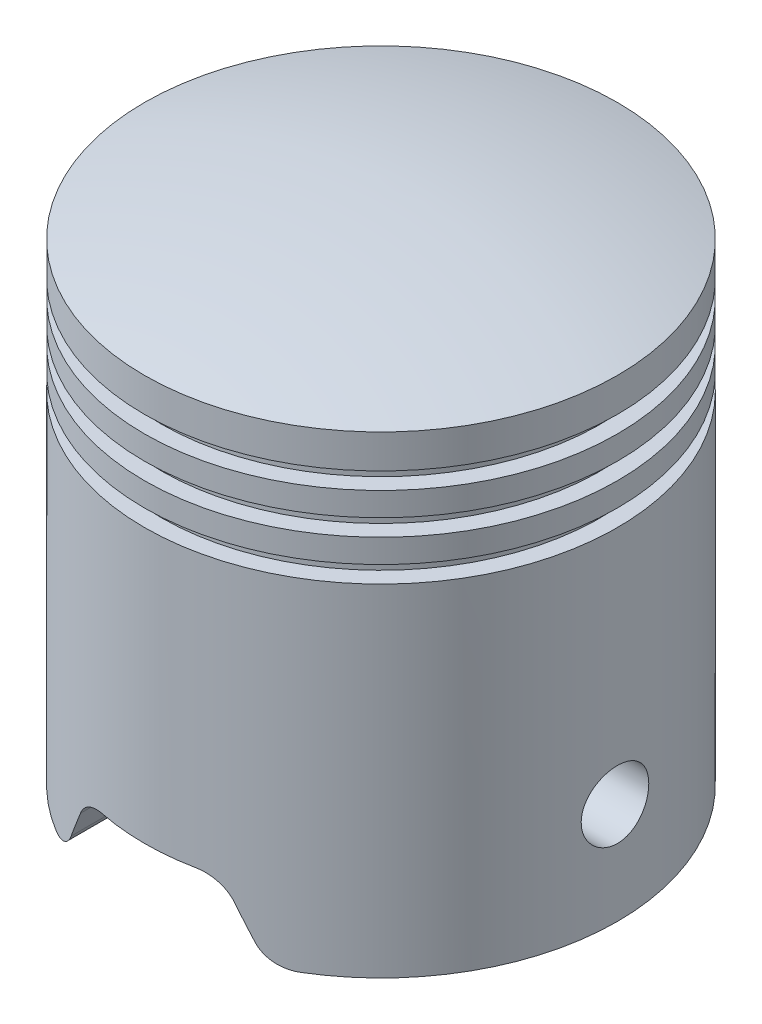
from build123d import *

# Parameters (mm, degrees)
PISTON_BODY_SKETCH_R       = 35
PISTON_BODY_70_DEPTH       = 35
RING_GROOVES_SKETCH_W      = 2.5
RING_GROOVES_SKETCH_H      = 2.5
INNER_BORE_SKETCH_R        = 29
INNER_BORE_58_DEPTH        = 65
SKIRT_CUTOUTS_DEPTH        = 61.621778265
SKIRT_CUTOUTS_DEPTH_BACK   = 61.621778265
SKIRT_CUTOUT_FILLET_R5_R   = 5
PIN_HOLE_10_DEPTH          = 61.621778438
PIN_HOLE_10_DEPTH_BACK     = 61.621778438
PIN_HOLE_SKETCH_R          = 5
PIN_BOSS_SKETCH_R          = 7.5
PIN_BOSS_15_DEPTH          = 32.5
PIN_BORE_DEPTH             = 84.703345378
PIN_BORE_DEPTH_BACK        = 84.703345378
PIN_BORE_SKETCH_R          = 5
CROWN_DOME_5MM_FACE_RADIUS = 35
CROWN_DOME_5MM_HEIGHT      = 5


with BuildPart() as part:
    # Piston Body Sketch → Piston Body _70 (new, symmetric)
    with BuildSketch(Plane(origin=(0, 0, 0), x_dir=(1, 0, 0), z_dir=(0, 1, 0))):
        with Locations(Location((0, 0, 0), (0, 0, 270))):
            Circle(PISTON_BODY_SKETCH_R)
    extrude(amount=PISTON_BODY_70_DEPTH, both=True)

    # Ring Grooves Sketch → Ring Grooves (revolve, cut)
    with BuildSketch(Plane(origin=(0, 0, 0), x_dir=(0, 0, -1), z_dir=(1, 0, 0))):
        with Locations((-33.75, 28.75)):
            Rectangle(RING_GROOVES_SKETCH_W, RING_GROOVES_SKETCH_H)
        with Locations((-33.75, 22.75)):
            Rectangle(RING_GROOVES_SKETCH_W, RING_GROOVES_SKETCH_H)
        with Locations((-33.75, 16.75)):
            Rectangle(RING_GROOVES_SKETCH_W, RING_GROOVES_SKETCH_H)
    revolve(axis=Axis((0, 35, 0), (0, -1, 0)), mode=Mode.SUBTRACT)

    # Inner Bore Sketch → Inner Bore _58 (cut)
    with BuildSketch(Plane.XZ.offset(35)):
        with Locations(Location((0, 0, 0), (0, 0, 270))):
            Circle(INNER_BORE_SKETCH_R)
    extrude(amount=-INNER_BORE_58_DEPTH, mode=Mode.SUBTRACT)

    # Skirt Cutout Sketch → Skirt Cutouts (cut, two sides: drawn at the far end of the back side and taken through both)
    with BuildSketch(Plane.XY.offset(-SKIRT_CUTOUTS_DEPTH_BACK)):
        with BuildLine():
            Line((15, -35), (-15, -35))
            Line((-15, -35), (-11.381966011, -27.763932023))
            ThreePointArc((-11.381966011, -27.763932023), (-9.538485617, -25.746745958), (-6.909830056, -25))
            Line((-6.909830056, -25), (6.909830056, -25))
            ThreePointArc((6.909830056, -25), (9.538485617, -25.746745958), (11.381966011, -27.763932023))
            Line((11.381966011, -27.763932023), (15, -35))
        make_face()
    extrude(amount=SKIRT_CUTOUTS_DEPTH + SKIRT_CUTOUTS_DEPTH_BACK, mode=Mode.SUBTRACT)

    # Skirt Cutout Fillet R5
    skirt_cutout_fillet_r5_edges = [part.edges().sort_by_distance(p)[0] for p in [
        (15, -35, -28.221061947),
        (15, -35, 28.221061947),
        (-15, -35, -28.221061947),
        (-15, -35, 28.221061947),
    ]]
    fillet(skirt_cutout_fillet_r5_edges, radius=SKIRT_CUTOUT_FILLET_R5_R)

    # Pin Hole Sketch → Pin Hole _10 (cut, two sides: drawn at the far end of the back side and taken through both)
    with BuildSketch(Plane(origin=(0, 0, 0), x_dir=(0, 0, -1), z_dir=(1, 0, 0)).offset(-PIN_HOLE_10_DEPTH_BACK)):
        with Locations((0, -20)):
            Circle(PIN_HOLE_SKETCH_R)
    extrude(amount=PIN_HOLE_10_DEPTH + PIN_HOLE_10_DEPTH_BACK, mode=Mode.SUBTRACT)

    # Pin Boss Sketch → Pin Boss _15 (add, symmetric)
    with BuildSketch(Plane(origin=(0, 0, 0), x_dir=(0, 0, -1), z_dir=(1, 0, 0))):
        with Locations(Location((0, -20, 0), (0, 0, 180))):
            Circle(PIN_BOSS_SKETCH_R)
    extrude(amount=PIN_BOSS_15_DEPTH, both=True)

    # Pin Bore Sketch → Pin Bore (cut, two sides: drawn at the far end of the back side and taken through both)
    with BuildSketch(Plane(origin=(32.5, 0, 0), x_dir=(0, 0, -1), z_dir=(1, 0, 0)).offset(-PIN_BORE_DEPTH_BACK)):
        with Locations((0, -20)):
            Circle(PIN_BORE_SKETCH_R)
    extrude(amount=PIN_BORE_DEPTH + PIN_BORE_DEPTH_BACK, mode=Mode.SUBTRACT)

    # Crown Dome 5mm: a dome of height H over a round flat face of radius A is a cap of a sphere of radius (A * A + H * H) / (2 * H)
    crown_dome_5mm_r = (CROWN_DOME_5MM_FACE_RADIUS * CROWN_DOME_5MM_FACE_RADIUS + CROWN_DOME_5MM_HEIGHT * CROWN_DOME_5MM_HEIGHT) / (2 * CROWN_DOME_5MM_HEIGHT)
    crown_dome_5mm_base = Plane((0, 35, 0), z_dir=(0, 1, 0))
    with Locations(crown_dome_5mm_base.offset(CROWN_DOME_5MM_HEIGHT - crown_dome_5mm_r)):
        crown_dome_5mm_ball = Sphere(crown_dome_5mm_r, mode=Mode.PRIVATE)
    add(split(crown_dome_5mm_ball, bisect_by=crown_dome_5mm_base, keep=Keep.TOP, mode=Mode.PRIVATE))


solid = part.part
